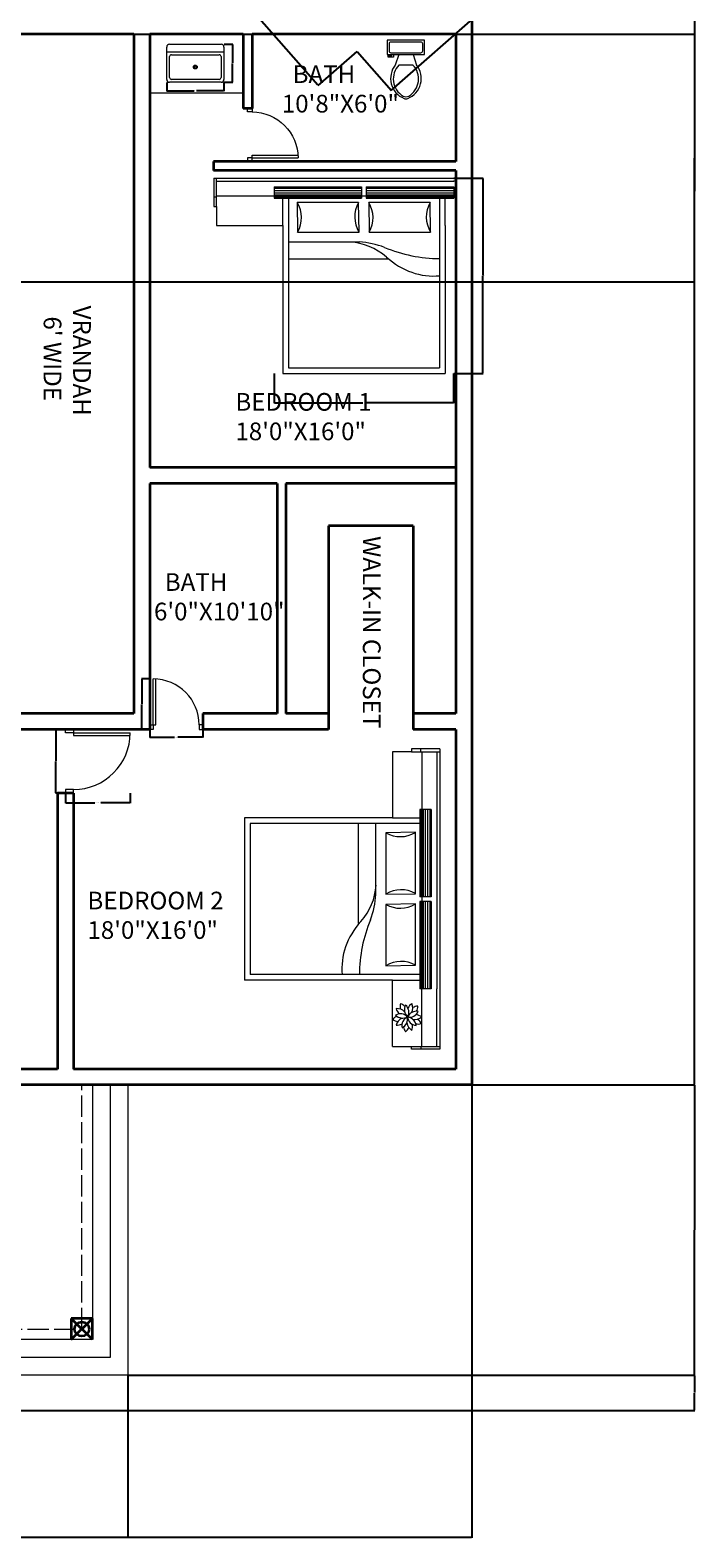
# Model space of a CAD drawing. Units: inches. Extents: x 4602 to 5612, y 5125 to 6591.
# Tile 3 of 6: x 5237 to 5612, y 5125 to 5977. Entities that reach past the tile are written whole.
import ezdxf

# ---------------------------------------------------------------- set-up
doc = ezdxf.new("R2010")
doc.units = ezdxf.units.IN
doc.linetypes.add('ACAD_ISO02W100', pattern=[15, 12, -3])
for name, color, linetype, lineweight in [('A-ANNO-DIMS', 2, 'Continuous', 18), ('A-AREA-IDEN', 7, 'Continuous', 18), ('A-COLS', 7, 'Continuous', 35), ('A-DOOR', 4, 'Continuous', 18), ('A-FLOR-CASE', 9, 'Continuous', 18), ('A-FLOR-EDGE', 7, 'Continuous', 18), ('A-FLOR-FIXT', 8, 'Continuous', 18), ('A-FLOR-OVHD', 8, 'ACAD_ISO02W100', 13), ('A-FLOR-STRS', 7, 'Continuous', 18), ('A-FURN', 8, 'Continuous', 13), ('A-WALL', 7, 'Continuous', 35)]:
    doc.layers.add(name, color=color, linetype=linetype, lineweight=lineweight)
doc.styles.add('ATTR', font='romans.shx', dxfattribs={"width": 0.8, "height": 1.075})
doc.styles.get("Standard").update_dxf_attribs({"font": 'arial.ttf'})
doc.dimstyles.get("Standard").update_dxf_attribs({"dimtxt": 0.18, "dimasz": 0.18, "dimexe": 0.18, "dimexo": 0.0625, "dimgap": 0.09, "dimtad": 0, "dimtih": 1, "dimtoh": 1, "dimdec": 4, "dimzin": 0, "dimdsep": 46, "dimtxsty": 'Standard', "dimcen": 0.09, "dimadec": 0, "dimazin": 0, "dimtfac": 1, "dimtdec": 4, "dimtofl": 0, "dimtmove": 0, "dimatfit": 3, "dimfxl": 1, "dimtolj": 1, "dimtzin": 0, "dimarcsym": 0})

# ---------------------------------------------------------------- blocks, each defined once
blk = doc.blocks.new('A$C25213C04')
for p, q in [((961, 2561), (805, 2831)), ((2063, 2927, 1584), (1415, 2360, 1584)), ((2063, 2927, 1584), (3697, 1495, 1584)), ((961, 2590), (805, 2320)), ((936, 2575), (1248, 2575)), ((2506, 2330, 1584), (2338, 2162, 1584)), ((2306, 2131, 1584), (2256, 2081, 1584)), ((3178, 1881), (3005, 2048)), ((2140, 1966, 1584), (2022, 1849, 1584)), ((1493, 1691), (720, 773)), ((2411, 918), (1493, 1691)), ((3026, 1811, 1584), (2854, 1589, 1584)), ((2839, 1570, 1584), (2748, 1452, 1584)), ((3697, 1495, 1584), (3220, 778, 1584)), ((2708, 1401, 1584), (2653, 1329, 1584)), ((3783, 1288), (3260, 764)), ((3783, 1245), (3302, 764)), ((4207, 863), (3783, 1288)), ((4165, 863), (3783, 1245)), ((720, 773), (1638, 0)), ((1638, 0), (2411, 918)), ((3260, 764), (3684, 340)), ((3302, 764), (3684, 382)), ((3684, 340), (4207, 863)), ((3684, 382), (4165, 863))]:
    blk.add_line(p, q)
at = {"linetype": 'ByBlock'}
for p, q in [((133, 1730), (136, 1691)), ((896, 1561), (877, 1527))]:
    blk.add_line(p, q, dxfattribs=at)
blk.add_lwpolyline([(725, 2173, -0.232884), (950, 2110, -0.135002), (887, 1960, -0.190823), (579, 2053, -0.215879), (600, 2250, -0.243587), (764, 2155, 4.263709)], format="xyb")
blk.add_lwpolyline([(472, 697, 0.343499), (533, 723, 0.070096), (548, 767, -0.063818), (573, 843, 0.079553), (601, 928, -0.057815), (620, 1007, 0.080725), (637, 1068, 0.324043), (600, 1120, -0.019241), (459, 1179, 0.08432), (309, 1223, -0.023422), (183, 1248, 0.070372), (146, 1253, 0.295986), (100, 1217, 0.032258), (86, 1168, -0.067929), (60, 1097, 0.081366), (35, 1016, -0.070774), (15, 936, 0.059814), (0, 885, 0.300433), (27, 833, 0.039992), (72, 815, -0.020153), (147, 783, 0.038402), (259, 739, 0.019707), (344, 722, -0.015856), (435, 705, 0.018827), (472, 697, 1.060826)], format="xyb", dxfattribs=at)
at = {"linetype": 'ByBlock', "flags": 128}
blk.add_lwpolyline([(324, 993, -1), (314, 960, -1)], format="xyb", close=True, dxfattribs=at)
blk.add_circle((953, 2575), 250)
for centre, radius, start, end in [((6904, 6804, 1584), 6250, 218.7122, 226.8714), ((6904, 6804, 1584), 6246, 218.7173, 226.8972), ((2075, 2768, 1584), 34.6, 301.5027, 35.2471), ((3283, 3449, 1584), 1352, 209.2555, 217.5058), ((2031, 2594, 1584), 222, 173.7702, 227.3147), ((1881, 2465, 1584), 169, 60.105, 114.9918), ((2065, 2440, 1584), 217, 75.8217, 128.2602), ((435, 4670, 1584), 2546, 306.4044, 310.6458), ((2178, 2539, 1584), 222, 167.7702, 221.3147), ((2015, 2427, 1584), 169, 54.105, 108.9918), ((2196, 2383, 1584), 217, 69.8217, 122.2602), ((1856, 2548, 1584), 282, 8.7006, 21.3114), ((1999, 2512, 1584), 282, 333.4414, 15.3114), ((742, 2652), 470, 213.6928, 250.0667), ((-111, -1286), 3707, 72.7192, 82.835), ((435, 4670, 1584), 2546, 293.2711, 302.9022), ((908, 3983, 1584), 1733, 288.4557, 300.3041), ((1986, 2631, 1584), 226, 242.3583, 273.8129), ((1838, 2738, 1584), 282, 280.859, 296.2171), ((2136, 2581, 1584), 226, 236.3583, 300.7775), ((1993, 2688, 1584), 282, 280.859, 322.7291), ((2044, 2704, 1584), 282, 271.8903, 313.7604), ((7978, 8701, 1584), 8396, 227.9717, 230.3292), ((-1544, 2942), 2094, 323.3441, 341.8043), ((590, 2045), 206, 32.2825, 87.042), ((742, 2652), 470, 270.1213, 301.8614), ((12303, 12967, 1584), 15201, 224.2521, 233.3075), ((3562, 3960, 1584), 2657, 217.5941, 222.0435), ((2720, 1975, 1584), 282, 105.7877, 147.6577), ((2508, 2077, 1584), 217, 358.839, 51.2774), ((591, 1710), 371, 44.935, 87.2084), ((487, 1559), 554, 48.4222, 73.8484), ((773, 1914), 264, 47.9991, 100.4376), ((2708, 2129, 1584), 226, 180.3216, 244.7408), ((2862, 2114, 1584), 282, 167.3388, 209.2088), ((2874, 2061, 1584), 282, 158.3701, 200.2401), ((6904, 6804, 1584), 6246, 227.5711, 228.2803), ((6904, 6804, 1584), 6250, 227.7194, 228.2519), ((2639, 1946, 1584), 169, 12.1073, 66.9941), ((7978, 8701, 1584), 8396, 231.1014, 231.3893), ((2825, 1872, 1584), 282, 99.7877, 112.3986), ((2625, 1995, 1584), 217, 352.839, 45.2774), ((2930, 1759, 1584), 282, 99.7877, 112.3986), ((6904, 6804, 1584), 6246, 229.2463, 229.7871), ((6904, 6804, 1584), 6250, 229.3273, 229.7524), ((8643, 8118, 1584), 8396, 226.2108, 226.4615), ((2730, 1883, 1584), 217, 352.839, 45.2774), ((10966, 12498, 1584), 13958, 229.1973, 231.6399), ((2651, 2143, 1584), 222, 259.7845, 313.329), ((2829, 2026, 1584), 226, 207.2862, 238.7408), ((2774, 2046, 1584), 222, 253.7845, 307.329), ((2997, 1955, 1584), 282, 184.882, 200.2401), ((2741, 1851, 1584), 169, 6.1073, 60.9941), ((6904, 6804, 1584), 6246, 230.2513, 238.8423), ((6904, 6804, 1584), 6250, 230.3855, 238.8474), ((2846, 1738, 1584), 169, 6.1073, 60.9941), ((8643, 8118, 1584), 8396, 227.1305, 229.5879), ((2934, 1914, 1584), 226, 201.8609, 238.7408), ((2879, 1934, 1584), 222, 253.7845, 307.329), ((3102, 1842, 1584), 282, 184.882, 200.2401), ((3294, 1377, 1584), 282, 82.2482, 124.1182), ((3140, 1555, 1584), 217, 335.2995, 27.7379), ((12014, 11580, 1584), 13958, 225.9197, 228.3623), ((3345, 1523, 1584), 226, 156.7821, 221.2013), ((3469, 1394, 1584), 282, 134.8306, 176.7006), ((3479, 1447, 1584), 282, 143.7993, 185.6693), ((3207, 1382, 1584), 169, 348.5678, 43.4546), ((3349, 1240, 1584), 282, 76.2482, 88.8591), ((4054, 2773, 1584), 1352, 240.0538, 248.3041), ((3214, 1433, 1584), 217, 329.2995, 21.7379), ((5640, 111, 1584), 2546, 146.9138, 151.1553), ((3538, 1486, 1584), 34.6, 62.3126, 156.0569), ((3298, 1558, 1584), 222, 236.2449, 289.7895), ((3414, 1380, 1584), 226, 183.7467, 215.2013), ((3539, 1247, 1584), 282, 161.3425, 176.7006), ((3263, 1255, 1584), 169, 342.5678, 37.4546), ((5640, 111, 1584), 2546, 154.6574, 164.2885), ((4896, 489, 1584), 1733, 157.2556, 169.1039), ((3372, 1420, 1584), 222, 230.2449, 283.7895), ((4524, 3117, 1584), 2657, 235.5161, 239.9655)]:
    blk.add_arc(centre, radius, start, end)
at = {"linetype": 'ByBlock'}
for centre, radius, start, end in [((3117, 1104), 3051, 155.0292, 167.8975), ((-2061, 2301), 3051, 346.2024, 359.1081), ((4037, 1940), 3187, 175.3548, 175.9684), ((4037, 1940), 3187, 179.6641, 187.4345), ((168, 1736), 35.5, 167.4303, 189.0652), ((187, 1686), 51, 173.5933, 247.766), ((1112, 4418), 2936, 251.2253, 257.771), ((1098, 4417), 2932, 258.0523, 264.7029), ((826, 1556), 57.8, 270.4071, 330.8661), ((867, 1581), 35.5, 325.0347, 346.6697), ((280, 872), 108, 80.0068, 116.3761), ((349, 1084), 108, 207.805, 244.1743), ((212, 1006), 108, 297.805, 334.1743), ((215, 1016), 108, 350.0068, 26.3761), ((424, 937), 108, 170.0068, 206.3761), ((427, 947), 108, 117.805, 154.1743), ((290, 869), 108, 27.805, 64.1743), ((358, 1081), 108, 260.0068, 296.3761)]:
    blk.add_arc(centre, radius, start, end, dxfattribs=at)
for major_axis, start_param, end_param in [((-153, 153), 3.927057, 7.06865), ((-64.8, 64.8), 3.927057, 7.06865), ((-153, 153), 0.785465, 3.927057), ((-64.8, 64.8), 0.785465, 3.927057)]:
    blk.add_ellipse((953, 2575), major_axis=major_axis, ratio=1, start_param=start_param, end_param=end_param)
blk = doc.blocks.new("30'' Sink Single PV")
blk.add_line((-15, -3.999996), (15, -3.999996))
for points in [[(-13.5, 0), (13.5, 0)], [(-15, -18.499996), (-15, -1.5)], [(-13.5, -17.499996), (-13.5, -6.499996)], [(-12.5, -5.499996), (12.5, -5.499996)], [(13.5, -6.499996), (13.5, -17.499996)], [(15, -1.5), (15, -18.499996)], [(13.5, -19.999996), (-13.5, -19.999996)], [(12.5, -18.499996), (-12.5, -18.499996)]]:
    blk.add_lwpolyline(points)
for radius in [1, 0.5]:
    blk.add_circle((0, -11.999996), radius)
for centre, radius, start, end in [((-13.5, -1.5), 1.5, 90, 180), ((-12.5, -6.499996), 1, 90, 180), ((12.5, -6.499996), 1, 0, 90), ((13.5, -1.5), 1.5, 0, 90), ((-13.5, -18.499996), 1.5, 180, 270), ((-12.5, -17.499996), 1, 180, 270), ((12.5, -17.499996), 1, 270, 0), ((13.5, -18.499996), 1.5, 270, 0)]:
    blk.add_arc(centre, radius, start, end)
at = {"style": 'ATTR', "width": 0.8, "flags": 9}
blk.add_attdef('ESTCODE', (0, 0), '', height=0.006, dxfattribs=at)
blk = doc.blocks.new('*U9')
for p, q in [((-254, -216), (-203, -216)), ((-254, -241), (-254, -216)), ((-203, -216), (-203, -203)), ((-178, -203), (-178, -241)), ((-102, -203), (-152, -356)), ((102, -203), (152, -356)), ((241, -152), (241, -51)), ((-178, -241), (-254, -241)), ((102, -356), (-102, -356))]:
    blk.add_line(p, q)
blk.add_lwpolyline([(267, -203), (267, 0), (-267, 0), (-267, -203)], close=True)
for points in [[(-241, -51), (-241, -152)], [(216, -25), (-216, -25)], [(-216, -178), (216, -178)]]:
    blk.add_lwpolyline(points)
for centre, radius, start, end in [((-219, -48), 22.5, 81.8699, 188.1301), ((-219, -156), 22.5, 171.8699, 278.1301), ((219, -48), 22.5, 351.8699, 98.1301), ((219, -156), 22.5, 261.8699, 8.1301), ((89, -548), 309, 141.4691, 247.9714), ((107, -554), 288, 136.3677, 238.9468), ((-89, -548), 309, 292.0284, 38.5307), ((-107, -554), 288, 301.053, 43.6321), ((0, -708), 102, 245.7318, 294.2682), ((0, -737), 102, 254.8605, 285.1395)]:
    blk.add_arc(centre, radius, start, end)
blk = doc.blocks.new('A$C7BDD1693')
for p, q in [((0, 2.068), (0, 1.768)), ((0, 2.068), (1.615, 2.068)), ((0.03, 1.768), (0.03, 2.068)), ((0.03, 2.038), (0.64, 2.038)), ((0.64, 2.038), (1.565, 2.038)), ((0.64, 1.978), (1.565, 1.978)), ((0.64, 1.978), (0.64, 1.858)), ((0.64, 1.963), (1.565, 1.963)), ((0.64, 1.937), (1.565, 1.937)), ((1.565, 2.038), (1.615, 2.038)), ((1.565, 1.978), (1.565, 1.858)), ((1.615, 2.068), (2.54, 2.068)), ((1.615, 2.038), (2.54, 2.038)), ((1.615, 1.978), (1.615, 1.858)), ((1.615, 1.978), (2.54, 1.978)), ((1.615, 1.963), (2.54, 1.963)), ((1.615, 1.937), (2.54, 1.937)), ((2.54, 2.068), (3.18, 2.068)), ((3.15, 2.038), (2.54, 2.038)), ((2.54, 1.978), (2.54, 1.858)), ((3.15, 1.768), (3.15, 2.068)), ((3.18, 2.068), (3.18, 1.768)), ((0.03, 1.868), (0, 1.868)), ((0, 1.768), (0.03, 1.768)), ((0.03, 1.88), (0.64, 1.88)), ((0.03, 1.768), (0.03, 1.568)), ((0.03, 1.768), (0.03, 1.568)), ((0.64, 1.912), (1.565, 1.912)), ((0.64, 1.893), (1.565, 1.893)), ((0.64, 1.877), (1.565, 1.877)), ((0.64, 1.866), (1.565, 1.866)), ((0.64, 1.858), (1.565, 1.858)), ((0.73, 1.568), (0.73, 1.858)), ((0.79, 1.858), (0.79, 0.06)), ((1.533, 1.81), (0.883, 1.81)), ((0.883, 1.81), (0.887, 1.498)), ((1.537, 1.498), (1.533, 1.81)), ((1.565, 1.88), (1.615, 1.88)), ((1.615, 1.912), (2.54, 1.912)), ((1.615, 1.893), (2.54, 1.893)), ((1.615, 1.877), (2.54, 1.877)), ((1.615, 1.866), (2.54, 1.866)), ((1.615, 1.858), (2.54, 1.858)), ((2.291, 1.81), (1.641, 1.81)), ((1.641, 1.81), (1.646, 1.498)), ((2.296, 1.498), (2.291, 1.81)), ((2.39, 1.858), (2.39, 0.06)), ((2.45, 1.568), (2.45, 1.858)), ((3.15, 1.88), (2.54, 1.88)), ((3.15, 1.868), (3.18, 1.868)), ((3.15, 1.568), (3.15, 1.768)), ((3.18, 1.768), (3.15, 1.768)), ((0.03, 1.568), (0.73, 1.568)), ((0.73, 1.568), (0.73, 0)), ((0.887, 1.498), (1.537, 1.498)), ((1.646, 1.498), (2.296, 1.498)), ((3.15, 1.568), (2.45, 1.568)), ((2.45, 1.568), (2.45, 0)), ((1.54, 1.392), (0.79, 1.392)), ((1.848, 1.209), (0.79, 1.209)), ((0.73, 0), (2.45, 0)), ((0.79, 0.06), (2.39, 0.06))]:
    blk.add_line(p, q)
for centre, radius, start, end in [((0.626, 1.65), 0.303, 329.8722, 31.8713), ((1.794, 1.658), 0.303, 149.8722, 211.8713), ((1.384, 1.65), 0.303, 329.8722, 31.8713), ((2.553, 1.658), 0.303, 149.8722, 211.8713), ((2.74, 1.667), 0.115, 63.1324, 112.6013), ((2.798, 1.845), 0.125, 215.1301, 245.4931), ((2.879, 1.849), 0.155, 184.2105, 205.3514), ((2.726, 1.74), 0.0968, 57.5086, 91.2476), ((2.884, 1.823), 0.106, 170.7761, 244.5159), ((2.743, 1.749), 0.098, 347.0447, 68.2473), ((2.938, 1.802), 0.125, 143.1301, 173.4932), ((2.751, 1.802), 0.115, 351.1324, 40.6013), ((2.944, 1.713), 0.106, 98.7761, 172.5159), ((2.83, 1.825), 0.098, 275.0447, 356.2473), ((2.967, 1.726), 0.155, 112.2105, 133.3514), ((2.883, 1.833), 0.115, 279.1324, 328.6013), ((2.817, 1.838), 0.0968, 345.5086, 19.2476), ((2.941, 1.655), 0.125, 71.1301, 101.4931), ((2.791, 1.624), 0.0968, 129.5086, 163.2476), ((2.735, 1.803), 0.155, 256.2105, 277.3514), ((2.788, 1.643), 0.098, 59.0447, 140.2473), ((2.761, 1.8), 0.106, 242.7761, 316.5159), ((2.865, 1.615), 0.115, 135.1324, 184.6013), ((2.713, 1.725), 0.125, 287.1301, 317.4932), ((2.903, 1.653), 0.098, 131.0447, 212.2473), ((2.745, 1.676), 0.106, 314.7761, 28.5159), ((2.921, 1.65), 0.0968, 201.5086, 235.2476), ((2.858, 1.622), 0.106, 26.7761, 100.5159), ((2.929, 1.765), 0.098, 203.0447, 284.2473), ((2.953, 1.718), 0.115, 207.1324, 256.6013), ((2.734, 1.652), 0.155, 328.2105, 349.3514), ((2.802, 1.607), 0.125, 359.1301, 29.4932), ((2.937, 1.782), 0.0968, 273.5086, 307.2476), ((2.877, 1.605), 0.155, 40.2105, 61.3514)]:
    blk.add_arc(centre, radius, start, end)
for centre, major_axis, ratio, start_param, end_param in [((1.413, 0.552), (0, -0.842), 0.84, 2.512571, 3.097265), ((1.474, 0.023), (0, -1.371), 0.84, 2.845884, 3.083884), ((2.394, 3.329), (0, -2.112), 0.84, -0.336035, -0.002349), ((2.261, 1.856), (0.259, -0.793), 0.868451, -0.988378, -0.183496)]:
    blk.add_ellipse(centre, major_axis=major_axis, ratio=ratio, start_param=start_param, end_param=end_param)
blk = doc.blocks.new('DOOR-36IN-DEEP-JAMB')
for p, q in [((2, 4.5), (2, 36.5)), ((3.5, 4.5), (3.5, 36.46)), ((0, 4.5), (2, 4.5)), ((2, 4.5), (2, 0)), ((2, 4.5), (3.5, 4.5)), ((36, 4.5), (34, 4.5)), ((34, 4.5), (34, 0)), ((2, 0), (0, 0)), ((34, 0), (36, 0))]:
    blk.add_line(p, q)
blk.add_arc((2, 4.5), 32, 0, 90)
blk = doc.blocks.new('DOOR-30IN')
for p, q in [((26, 30), (26, 28)), ((26, 28), (28.5, 28)), ((28.5, 28), (28.5, 30)), ((26, 2), (0, 2)), ((26, 3.5), (0.04, 3.5)), ((26, 2), (26, 3.5)), ((26, 0), (26, 2)), ((26, 2), (28.5, 2)), ((28.5, 2), (28.5, 0))]:
    blk.add_line(p, q)
blk.add_arc((26, 2), 26, 90, 180)
blk = doc.blocks.new('POST-POOMUKHAM')
for p, q in [((12, 12), (0, 12)), ((0, 12), (0, 0)), ((12, 0), (0, 12)), ((0, 0), (12, 12)), ((12, 0), (12, 12))]:
    blk.add_line(p, q)
blk.add_circle((6, 6), 4.06)
blk = doc.blocks.new('BED-DOUBLE')
for p, q in [((0, 108.76), (49.36, 108.76)), ((0, 105.55), (49.36, 105.55)), ((0, 105.55), (0, 99.15)), ((0, 104.75), (49.36, 104.75)), ((0, 103.35), (49.36, 103.35)), ((49.36, 108.76), (52.03, 108.76)), ((49.36, 105.55), (49.36, 99.15)), ((52.03, 110.36), (101.4, 110.36)), ((52.03, 108.76), (101.4, 108.76)), ((52.03, 105.55), (52.03, 99.15)), ((52.03, 105.55), (101.4, 105.55)), ((52.03, 104.75), (101.4, 104.75)), ((52.03, 103.35), (101.4, 103.35)), ((101.4, 105.55), (101.4, 99.15)), ((0, 102.06), (49.36, 102.06)), ((0, 101), (49.36, 101)), ((0, 100.18), (49.36, 100.18)), ((0, 99.59), (49.36, 99.59)), ((0, 99.15), (49.36, 99.15)), ((4.8, 83.67), (4.8, 99.15)), ((8.01, 99.15), (8.01, 3.2)), ((47.64, 96.58), (12.95, 96.58)), ((12.95, 96.58), (13.21, 79.95)), ((47.9, 79.95), (47.64, 96.58)), ((49.36, 100.32), (52.03, 100.32)), ((52.03, 102.06), (101.4, 102.06)), ((52.03, 101), (101.4, 101)), ((52.03, 100.18), (101.4, 100.18)), ((52.03, 99.59), (101.4, 99.59)), ((52.03, 99.15), (101.4, 99.15)), ((88.11, 96.58), (53.42, 96.58)), ((53.42, 96.58), (53.67, 79.95)), ((88.36, 79.95), (88.11, 96.58)), ((93.39, 99.15), (93.39, 3.2)), ((96.59, 83.67), (96.59, 99.15)), ((4.8, 83.67), (4.8, 0)), ((13.21, 79.95), (47.9, 79.95)), ((53.67, 79.95), (88.36, 79.95)), ((96.59, 83.67), (96.59, 0)), ((48.03, 74.3), (8.01, 74.3)), ((64.45, 64.53), (8.01, 64.53)), ((4.8, 0), (96.59, 0)), ((8.01, 3.2), (93.39, 3.2))]:
    blk.add_line(p, q)
for centre, start, end in [((-0.76, 88.06), 329.87223, 31.87128), ((61.61, 88.48), 149.87223, 211.87128), ((39.71, 88.06), 329.87223, 31.87128), ((102.07, 88.48), 149.87223, 211.87128)]:
    blk.add_arc(centre, 16.15, start, end)
for centre, major_axis, ratio, start_param, end_param in [((41.23, 29.43), (0, -44.91), 0.84, 2.512571, 3.097265), ((44.48, 1.25), (0, -73.18), 0.84, 2.845884, 3.083884), ((93.61, 177.65), (0, -112.7), 0.84, -0.336035, -0.002349), ((86.52, 99.05), (13.81, -42.31), 0.868451, -0.988378, -0.183496)]:
    blk.add_ellipse(centre, major_axis=major_axis, ratio=ratio, start_param=start_param, end_param=end_param)
blk = doc.blocks.new('*D23')
at = {"layer": 'A-ANNO-DIMS', "color": 0, "lineweight": -2, "transparency": 16777216}
for p, q in [((5256.74, 5545.49), (5256.74, 5539.9)), ((5256.92, 5540.08), (5273.3, 5540.08)), ((5293.06, 5540.08), (5276.68, 5540.08)), ((5293.24, 5545.49), (5293.24, 5539.9))]:
    blk.add_line(p, q, dxfattribs=at)
at = {"layer": 'A-ANNO-DIMS', "color": 0, "transparency": 16777216}
for points in [[(5256.92, 5540.11), (5256.92, 5540.05), (5256.74, 5540.08)], [(5293.06, 5540.11), (5293.06, 5540.05), (5293.24, 5540.08)]]:
    blk.add_solid(points, dxfattribs=at)
at = {"layer": 'Defpoints', "color": 0, "transparency": 16777216}
for p in [(5256.74, 5545.55), (5293.24, 5545.55), (5293.24, 5540.08)]:
    blk.add_point(p, dxfattribs=at)
at = {"layer": 'A-ANNO-DIMS', "color": 0, "transparency": 16777216, "insert": (5274.99, 5540.08), "char_height": 0.18, "attachment_point": 5}
blk.add_mtext('\\A1;DEEP-JAMB DOOR 37 TYP.', dxfattribs=at)
blk = doc.blocks.new('*D24')
at = {"layer": 'A-ANNO-DIMS', "color": 0, "lineweight": -2, "transparency": 16777216}
for p, q in [((5256.68, 5581.55), (5251.08, 5581.55)), ((5251.26, 5581.37), (5251.26, 5563.73)), ((5251.26, 5545.73), (5251.26, 5563.37)), ((5256.68, 5545.55), (5251.08, 5545.55))]:
    blk.add_line(p, q, dxfattribs=at)
at = {"layer": 'A-ANNO-DIMS', "color": 0, "transparency": 16777216}
for points in [[(5251.23, 5581.37), (5251.29, 5581.37), (5251.26, 5581.55)], [(5251.23, 5545.73), (5251.29, 5545.73), (5251.26, 5545.55)]]:
    blk.add_solid(points, dxfattribs=at)
at = {"layer": 'Defpoints', "color": 0, "transparency": 16777216}
for p in [(5256.74, 5581.55), (5251.26, 5545.55), (5256.74, 5545.55)]:
    blk.add_point(p, dxfattribs=at)
at = {"layer": 'A-ANNO-DIMS', "color": 0, "transparency": 16777216, "insert": (5251.26, 5563.55), "char_height": 0.18, "attachment_point": 5}
blk.add_mtext('\\A1;36 TYP.', dxfattribs=at)
blk = doc.blocks.new('*D27')
at = {"layer": 'A-ANNO-DIMS', "color": 0, "lineweight": -2, "transparency": 16777216}
for p, q in [((5304.24, 5581.49), (5304.24, 5576.87)), ((5304.42, 5577.05), (5318.3, 5577.05)), ((5334.06, 5577.05), (5320.17, 5577.05)), ((5334.24, 5581.49), (5334.24, 5576.87))]:
    blk.add_line(p, q, dxfattribs=at)
at = {"layer": 'A-ANNO-DIMS', "color": 0, "transparency": 16777216}
for points in [[(5304.42, 5577.08), (5304.42, 5577.02), (5304.24, 5577.05)], [(5334.06, 5577.08), (5334.06, 5577.02), (5334.24, 5577.05)]]:
    blk.add_solid(points, dxfattribs=at)
at = {"layer": 'Defpoints', "color": 0, "transparency": 16777216}
for p in [(5304.24, 5581.55), (5334.24, 5581.55), (5334.24, 5577.05)]:
    blk.add_point(p, dxfattribs=at)
at = {"layer": 'A-ANNO-DIMS', "color": 0, "transparency": 16777216, "insert": (5319.24, 5577.05), "char_height": 0.18, "attachment_point": 5}
blk.add_mtext('\\A1;DOOR 30 TYP.', dxfattribs=at)
blk = doc.blocks.new('*D28')
at = {"layer": 'A-ANNO-DIMS', "color": 0, "lineweight": -2, "transparency": 16777216}
for p, q in [((5304.18, 5610.05), (5299.56, 5610.05)), ((5299.74, 5609.87), (5299.74, 5595.98)), ((5299.74, 5581.73), (5299.74, 5595.62)), ((5304.18, 5581.55), (5299.56, 5581.55))]:
    blk.add_line(p, q, dxfattribs=at)
at = {"layer": 'A-ANNO-DIMS', "color": 0, "transparency": 16777216}
for points in [[(5299.71, 5609.87), (5299.77, 5609.87), (5299.74, 5610.05)], [(5299.71, 5581.73), (5299.77, 5581.73), (5299.74, 5581.55)]]:
    blk.add_solid(points, dxfattribs=at)
at = {"layer": 'Defpoints', "color": 0, "transparency": 16777216}
for p in [(5304.24, 5610.05), (5299.74, 5581.55), (5304.24, 5581.55)]:
    blk.add_point(p, dxfattribs=at)
at = {"layer": 'A-ANNO-DIMS', "color": 0, "transparency": 16777216, "insert": (5299.74, 5595.8), "char_height": 0.18, "attachment_point": 5}
blk.add_mtext('\\A1;29 TYP.', dxfattribs=at)
blk = doc.blocks.new('*D37')
at = {"layer": 'A-ANNO-DIMS', "color": 0, "lineweight": -2, "transparency": 16777216}
for p, q in [((5476.11, 5893.1), (5492.78, 5893.1)), ((5492.6, 5892.92), (5492.6, 5838.11)), ((5492.6, 5782.93), (5492.6, 5837.74)), ((5476.11, 5782.75), (5492.78, 5782.75))]:
    blk.add_line(p, q, dxfattribs=at)
at = {"layer": 'A-ANNO-DIMS', "color": 0, "transparency": 16777216}
for points in [[(5492.57, 5892.92), (5492.63, 5892.92), (5492.6, 5893.1)], [(5492.57, 5782.93), (5492.63, 5782.93), (5492.6, 5782.75)]]:
    blk.add_solid(points, dxfattribs=at)
at = {"layer": 'Defpoints', "color": 0, "transparency": 16777216}
for p in [(5476.05, 5893.1), (5492.6, 5893.1), (5476.05, 5782.75)]:
    blk.add_point(p, dxfattribs=at)
at = {"layer": 'A-ANNO-DIMS', "color": 0, "transparency": 16777216, "insert": (5492.6, 5837.92), "char_height": 0.18, "attachment_point": 5}
blk.add_mtext('\\A1;DOUBLE BED 110 TYP.', dxfattribs=at)
blk = doc.blocks.new('*D38')
at = {"layer": 'A-ANNO-DIMS', "color": 0, "lineweight": -2, "transparency": 16777216}
for p, q in [((5374.65, 5782.68), (5374.65, 5766.01)), ((5476.05, 5782.68), (5476.05, 5766.01)), ((5374.83, 5766.19), (5424.76, 5766.19)), ((5475.87, 5766.19), (5425.94, 5766.19))]:
    blk.add_line(p, q, dxfattribs=at)
at = {"layer": 'A-ANNO-DIMS', "color": 0, "transparency": 16777216}
for points in [[(5374.83, 5766.22), (5374.83, 5766.16), (5374.65, 5766.19)], [(5475.87, 5766.22), (5475.87, 5766.16), (5476.05, 5766.19)]]:
    blk.add_solid(points, dxfattribs=at)
at = {"layer": 'Defpoints', "color": 0, "transparency": 16777216}
for p in [(5374.65, 5782.75), (5476.05, 5782.75), (5476.05, 5766.19)]:
    blk.add_point(p, dxfattribs=at)
at = {"layer": 'A-ANNO-DIMS', "color": 0, "transparency": 16777216, "insert": (5425.35, 5766.19), "char_height": 0.18, "attachment_point": 5}
blk.add_mtext('\\A1;101 TYP.', dxfattribs=at)
blk = doc.blocks.new('*D43')
at = {"layer": 'A-ANNO-DIMS', "color": 0, "lineweight": -2, "transparency": 16777216}
for p, q in [((5313.85, 5947.25), (5313.85, 5942.28)), ((5314.03, 5942.46), (5329.4, 5942.46)), ((5346.01, 5942.46), (5330.65, 5942.46)), ((5346.19, 5947.25), (5346.19, 5942.28))]:
    blk.add_line(p, q, dxfattribs=at)
at = {"layer": 'A-ANNO-DIMS', "color": 0, "transparency": 16777216}
for points in [[(5314.03, 5942.49), (5314.03, 5942.43), (5313.85, 5942.46)], [(5346.01, 5942.49), (5346.01, 5942.43), (5346.19, 5942.46)]]:
    blk.add_solid(points, dxfattribs=at)
at = {"layer": 'Defpoints', "color": 0, "transparency": 16777216}
for p in [(5313.85, 5947.31), (5346.19, 5947.31), (5346.19, 5942.46)]:
    blk.add_point(p, dxfattribs=at)
at = {"layer": 'A-ANNO-DIMS', "color": 0, "transparency": 16777216, "insert": (5330.02, 5942.46), "char_height": 0.18, "attachment_point": 5}
blk.add_mtext('\\A1;BASIN 32', dxfattribs=at)
blk = doc.blocks.new('*D44')
at = {"layer": 'A-ANNO-DIMS', "color": 0, "lineweight": -2, "transparency": 16777216}
for p, q in [((5346.25, 5968.87), (5351.22, 5968.87)), ((5351.04, 5968.69), (5351.04, 5958.27)), ((5351.04, 5947.49), (5351.04, 5957.91)), ((5346.25, 5947.31), (5351.22, 5947.31))]:
    blk.add_line(p, q, dxfattribs=at)
at = {"layer": 'A-ANNO-DIMS', "color": 0, "transparency": 16777216}
for points in [[(5351.01, 5968.69), (5351.07, 5968.69), (5351.04, 5968.87)], [(5351.01, 5947.49), (5351.07, 5947.49), (5351.04, 5947.31)]]:
    blk.add_solid(points, dxfattribs=at)
at = {"layer": 'Defpoints', "color": 0, "transparency": 16777216}
for p in [(5346.19, 5968.87), (5351.04, 5968.87), (5346.19, 5947.31)]:
    blk.add_point(p, dxfattribs=at)
at = {"layer": 'A-ANNO-DIMS', "color": 0, "transparency": 16777216, "insert": (5351.04, 5958.09), "char_height": 0.18, "attachment_point": 5}
blk.add_mtext('\\A1;22', dxfattribs=at)
blk = doc.blocks.new('*D49')
at = {"layer": 'A-ANNO-DIMS', "color": 0, "lineweight": -2, "transparency": 16777216}
for p, q in [((5293.01, 6111.54), (5270.91, 6092.21)), ((5271.16, 6092.19), (5335.08, 6019.13)), ((5399.32, 5945.7), (5335.4, 6018.76)), ((5421.4, 5964.78), (5399.3, 5945.45))]:
    blk.add_line(p, q, dxfattribs=at)
at = {"layer": 'A-ANNO-DIMS', "color": 0, "transparency": 16777216}
for points in [[(5271.18, 6092.21), (5271.14, 6092.17), (5271.04, 6092.33)], [(5399.34, 5945.72), (5399.29, 5945.68), (5399.43, 5945.57)]]:
    blk.add_solid(points, dxfattribs=at)
at = {"layer": 'Defpoints', "color": 0, "transparency": 16777216}
for p in [(5293.05, 6111.58), (5421.45, 5964.83), (5399.43, 5945.57)]:
    blk.add_point(p, dxfattribs=at)
at = {"layer": 'A-ANNO-DIMS', "color": 0, "transparency": 16777216, "insert": (5335.24, 6018.95), "char_height": 0.18, "attachment_point": 5}
blk.add_mtext('\\A1;FAMILY SEATING 195', dxfattribs=at)
blk = doc.blocks.new('*D50')
at = {"layer": 'A-ANNO-DIMS', "color": 0, "lineweight": -2, "transparency": 16777216}
for p, q in [((5523.54, 6054.06), (5542.88, 6031.96)), ((5542.62, 6031.97), (5491.94, 5987.63)), ((5440.84, 5942.93), (5491.53, 5987.27)), ((5421.49, 5964.78), (5440.83, 5942.68))]:
    blk.add_line(p, q, dxfattribs=at)
at = {"layer": 'A-ANNO-DIMS', "color": 0, "transparency": 16777216}
for points in [[(5542.6, 6032), (5542.64, 6031.95), (5542.76, 6032.09)], [(5440.82, 5942.95), (5440.86, 5942.91), (5440.71, 5942.81)]]:
    blk.add_solid(points, dxfattribs=at)
at = {"layer": 'Defpoints', "color": 0, "transparency": 16777216}
for p in [(5523.5, 6054.11), (5542.76, 6032.09), (5421.45, 5964.83)]:
    blk.add_point(p, dxfattribs=at)
at = {"layer": 'A-ANNO-DIMS', "color": 0, "transparency": 16777216, "insert": (5491.73, 5987.45), "char_height": 0.18, "attachment_point": 5}
blk.add_mtext('\\A1;136', dxfattribs=at)
blk = doc.blocks.new('*D57')
at = {"layer": 'A-ANNO-DIMS', "color": 0, "lineweight": -2, "transparency": 16777216}
for p, q in [((4720.24, 5380.49), (4720.24, 5124.52)), ((5486.24, 5380.49), (5486.24, 5124.52)), ((4720.42, 5124.7), (5102.95, 5124.7)), ((5486.06, 5124.7), (5103.53, 5124.7))]:
    blk.add_line(p, q, dxfattribs=at)
at = {"layer": 'A-ANNO-DIMS', "color": 0, "transparency": 16777216}
for points in [[(4720.42, 5124.73), (4720.42, 5124.67), (4720.24, 5124.7)], [(5486.06, 5124.73), (5486.06, 5124.67), (5486.24, 5124.7)]]:
    blk.add_solid(points, dxfattribs=at)
at = {"layer": 'Defpoints', "color": 0, "transparency": 16777216}
for p in [(4720.24, 5380.55), (5486.24, 5380.55), (5486.24, 5124.7)]:
    blk.add_point(p, dxfattribs=at)
at = {"layer": 'A-ANNO-DIMS', "color": 0, "transparency": 16777216, "insert": (5103.24, 5124.7), "char_height": 0.18, "attachment_point": 5}
blk.add_mtext('\\A1;766', dxfattribs=at)
blk = doc.blocks.new('*D58')
at = {"layer": 'A-ANNO-DIMS', "color": 0, "lineweight": -2, "transparency": 16777216}
for p, q in [((5486.3, 6390.55), (5612.27, 6390.55)), ((5612.09, 6390.37), (5612.09, 5885.73)), ((5612.09, 5380.73), (5612.09, 5885.37)), ((5486.3, 5380.55), (5612.27, 5380.55))]:
    blk.add_line(p, q, dxfattribs=at)
at = {"layer": 'A-ANNO-DIMS', "color": 0, "transparency": 16777216}
for points in [[(5612.06, 6390.37), (5612.12, 6390.37), (5612.09, 6390.55)], [(5612.06, 5380.73), (5612.12, 5380.73), (5612.09, 5380.55)]]:
    blk.add_solid(points, dxfattribs=at)
at = {"layer": 'Defpoints', "color": 0, "transparency": 16777216}
for p in [(5486.24, 6390.55), (5612.09, 6390.55), (5486.24, 5380.55)]:
    blk.add_point(p, dxfattribs=at)
at = {"layer": 'A-ANNO-DIMS', "color": 0, "transparency": 16777216, "insert": (5612.09, 5885.55), "char_height": 0.18, "attachment_point": 5}
blk.add_mtext('\\A1;1010', dxfattribs=at)
blk = doc.blocks.new('*D64')
at = {"layer": 'A-ANNO-DIMS', "color": 0, "lineweight": -2, "transparency": 16777216}
for p, q in [((4860.3, 5974.55), (5612.27, 5974.55)), ((5612.09, 5974.37), (5612.09, 5904.73)), ((5612.09, 5834.73), (5612.09, 5904.37)), ((4860.3, 5834.55), (5612.27, 5834.55))]:
    blk.add_line(p, q, dxfattribs=at)
at = {"layer": 'A-ANNO-DIMS', "color": 0, "transparency": 16777216}
for points in [[(5612.06, 5974.37), (5612.12, 5974.37), (5612.09, 5974.55)], [(5612.06, 5834.73), (5612.12, 5834.73), (5612.09, 5834.55)]]:
    blk.add_solid(points, dxfattribs=at)
at = {"layer": 'Defpoints', "color": 0, "transparency": 16777216}
for p in [(4860.24, 5974.55), (5612.09, 5974.55), (4860.24, 5834.55)]:
    blk.add_point(p, dxfattribs=at)
at = {"layer": 'A-ANNO-DIMS', "color": 0, "transparency": 16777216, "insert": (5612.09, 5904.55), "char_height": 0.18, "attachment_point": 5}
blk.add_mtext('\\A1;140', dxfattribs=at)
blk = doc.blocks.new('*D65')
at = {"layer": 'A-ANNO-DIMS', "color": 0, "lineweight": -2, "transparency": 16777216}
for p, q in [((4914.59, 5216.49), (4914.59, 5124.52)), ((5291.89, 5216.49), (5291.89, 5124.52)), ((4914.77, 5124.7), (5102.85, 5124.7)), ((5291.71, 5124.7), (5103.63, 5124.7))]:
    blk.add_line(p, q, dxfattribs=at)
at = {"layer": 'A-ANNO-DIMS', "color": 0, "transparency": 16777216}
for points in [[(4914.77, 5124.73), (4914.77, 5124.67), (4914.59, 5124.7)], [(5291.71, 5124.73), (5291.71, 5124.67), (5291.89, 5124.7)]]:
    blk.add_solid(points, dxfattribs=at)
at = {"layer": 'Defpoints', "color": 0, "transparency": 16777216}
for p in [(4914.59, 5216.55), (5291.89, 5216.55), (5291.89, 5124.7)]:
    blk.add_point(p, dxfattribs=at)
at = {"layer": 'A-ANNO-DIMS', "color": 0, "transparency": 16777216, "insert": (5103.24, 5124.7), "char_height": 0.18, "attachment_point": 5}
blk.add_mtext('\\A1;377.3', dxfattribs=at)
blk = doc.blocks.new('*D66')
at = {"layer": 'A-ANNO-DIMS', "color": 0, "lineweight": -2, "transparency": 16777216}
for p, q in [((5291.95, 5380.55), (5612.27, 5380.55)), ((5612.09, 5380.37), (5612.09, 5298.73)), ((5612.09, 5216.73), (5612.09, 5298.37)), ((5291.95, 5216.55), (5612.27, 5216.55))]:
    blk.add_line(p, q, dxfattribs=at)
at = {"layer": 'A-ANNO-DIMS', "color": 0, "transparency": 16777216}
for points in [[(5612.06, 5380.37), (5612.12, 5380.37), (5612.09, 5380.55)], [(5612.06, 5216.73), (5612.12, 5216.73), (5612.09, 5216.55)]]:
    blk.add_solid(points, dxfattribs=at)
at = {"layer": 'Defpoints', "color": 0, "transparency": 16777216}
for p in [(5291.89, 5380.55), (5612.09, 5380.55), (5291.89, 5216.55)]:
    blk.add_point(p, dxfattribs=at)
at = {"layer": 'A-ANNO-DIMS', "color": 0, "transparency": 16777216, "insert": (5612.09, 5298.55), "char_height": 0.18, "attachment_point": 5}
blk.add_mtext('\\A1;164', dxfattribs=at)
blk = doc.blocks.new('*D68')
at = {"layer": 'A-ANNO-DIMS', "color": 0, "lineweight": -2, "transparency": 16777216}
for p, q in [((5291.95, 5216.55), (5612.27, 5216.55)), ((5612.09, 5216.37), (5612.09, 5206.73)), ((5612.09, 5196.73), (5612.09, 5206.37)), ((5151.3, 5196.55), (5612.27, 5196.55))]:
    blk.add_line(p, q, dxfattribs=at)
at = {"layer": 'A-ANNO-DIMS', "color": 0, "transparency": 16777216}
for points in [[(5612.06, 5216.37), (5612.12, 5216.37), (5612.09, 5216.55)], [(5612.06, 5196.73), (5612.12, 5196.73), (5612.09, 5196.55)]]:
    blk.add_solid(points, dxfattribs=at)
at = {"layer": 'Defpoints', "color": 0, "transparency": 16777216}
for p in [(5291.89, 5216.55), (5612.09, 5216.55), (5151.24, 5196.55)]:
    blk.add_point(p, dxfattribs=at)
at = {"layer": 'A-ANNO-DIMS', "color": 0, "transparency": 16777216, "insert": (5612.09, 5206.55), "char_height": 0.18, "attachment_point": 5}
blk.add_mtext('\\A1;20', dxfattribs=at)

msp = doc.modelspace()

# ---------------------------------------------------------------- linework, layer by layer
at = {"layer": 'A-FLOR-CASE'}
msp.add_line((5357.1023, 5941.1104), (5304.239, 5941.1104), dxfattribs=at)
at = {"layer": 'A-FLOR-EDGE'}
for p, q in [((5271.8903, 5380.5515), (5271.8903, 5236.5515)), ((5271.8903, 5236.5515), (4934.5878, 5236.5515))]:
    msp.add_line(p, q, dxfattribs=at)
at = {"layer": 'A-FLOR-OVHD'}
for p, q in [((5265.8903, 5242.5515), (5265.8903, 5380.5515)), ((5145.239, 5242.5515), (5265.8903, 5242.5515))]:
    msp.add_line(p, q, dxfattribs=at)
at = {"layer": 'A-FLOR-STRS'}
for p, q in [((5281.8903, 5380.5515), (5281.8903, 5226.5515)), ((5291.8903, 5380.5515), (5291.8903, 5216.5515)), ((5281.8903, 5226.5515), (5151.239, 5226.5515)), ((5291.8903, 5216.5515), (5151.239, 5216.5515))]:
    msp.add_line(p, q, dxfattribs=at)
at = {"layer": 'A-FURN'}
for p, q in [((5340.4995, 5893.1022), (5340.4995, 5877.0923)), ((5340.4995, 5893.1022), (5426.6865, 5893.1022)), ((5342.1005, 5877.0923), (5342.1005, 5893.1022)), ((5342.1005, 5891.5012), (5374.6541, 5891.5012)), ((5476.0505, 5893.1022), (5477.239, 5893.1022)), ((5477.239, 5891.5012), (5476.0505, 5891.5012)), ((5342.1005, 5882.4289), (5340.4995, 5882.4289)), ((5342.1005, 5883.0693), (5374.6541, 5883.0693)), ((5340.4995, 5877.0923), (5342.1005, 5877.0923)), ((5342.1005, 5877.0923), (5342.1005, 5866.4189)), ((5342.1005, 5877.0923), (5342.1005, 5866.4189)), ((5342.1005, 5866.4189), (5379.4571, 5866.4189))]:
    msp.add_line(p, q, dxfattribs=at)
at = {"layer": 'A-WALL'}
for p, q in [((5486.239, 6051.5515), (5486.239, 5974.5515)), ((5295.239, 5974.5515), (5110.739, 5974.5515)), ((5295.239, 5974.5515), (5295.239, 5590.5515)), ((5304.239, 5974.5515), (5304.239, 5729.5515)), ((5357.1023, 5974.5515), (5304.239, 5974.5515)), ((5357.1023, 5974.5515), (5357.1023, 5932.5515)), ((5477.239, 5974.5515), (5362.1023, 5974.5515)), ((5362.1023, 5974.5515), (5362.1023, 5932.5515)), ((5477.239, 5974.5515), (5477.239, 5902.5515)), ((5486.239, 5974.5515), (5486.239, 5380.5515)), ((5362.1023, 5932.5515), (5357.1023, 5932.5515)), ((5357.1023, 5902.5515), (5340.239, 5902.5515)), ((5340.239, 5902.5515), (5340.239, 5897.5515)), ((5477.239, 5902.5515), (5357.1023, 5902.5515)), ((5477.239, 5897.5515), (5340.239, 5897.5515)), ((5477.239, 5897.5515), (5477.239, 5590.5515)), ((5477.239, 5729.5515), (5304.239, 5729.5515)), ((5376.239, 5720.5515), (5304.239, 5720.5515)), ((5304.239, 5720.5515), (5304.239, 5581.5515)), ((5376.239, 5720.5515), (5376.239, 5590.5515)), ((5477.239, 5720.5515), (5381.239, 5720.5515)), ((5381.239, 5720.5515), (5381.239, 5590.5515)), ((5405.239, 5696.5515), (5405.239, 5581.5515)), ((5453.239, 5696.5515), (5405.239, 5696.5515)), ((5453.239, 5696.5515), (5453.239, 5581.5515)), ((5295.239, 5590.5515), (5133.239, 5590.5515)), ((5376.239, 5590.5515), (5334.239, 5590.5515)), ((5334.239, 5590.5515), (5334.239, 5581.5515)), ((5405.239, 5590.5515), (5381.239, 5590.5515)), ((5477.239, 5590.5515), (5453.239, 5590.5515)), ((5304.239, 5581.5515), (5133.239, 5581.5515)), ((5405.239, 5581.5515), (5334.239, 5581.5515)), ((5477.239, 5581.5515), (5453.239, 5581.5515)), ((5477.239, 5581.5515), (5477.239, 5389.5515)), ((5252.239, 5545.5515), (5252.239, 5389.5515)), ((5261.239, 5545.5515), (5252.239, 5545.5515)), ((5261.239, 5545.5515), (5261.239, 5389.5515)), ((5252.239, 5389.5515), (5133.239, 5389.5515)), ((5477.239, 5389.5515), (5261.239, 5389.5515)), ((5486.239, 5380.5515), (5133.239, 5380.5515))]:
    msp.add_line(p, q, dxfattribs=at)

# ---------------------------------------------------------------- block references
at = {"layer": 'A-COLS'}
msp.add_blockref('POST-POOMUKHAM', (5259.8903, 5236.552), dxfattribs=at)
at = {"layer": 'A-DOOR', "extrusion": (0, 0, -1), "zscale": -1}
msp.add_blockref('DOOR-30IN', (-5388.1023, 5902.552), dxfattribs=at)
at = {"layer": 'A-DOOR'}
for name, p, rotation in [('DOOR-30IN', (5304.2395, 5610.0516), 269.9999999999796), ('DOOR-36IN-DEEP-JAMB', (5256.7395, 5581.5516), 269.9999999999988)]:
    msp.add_blockref(name, p, dxfattribs=dict(at, rotation=rotation))
at = {"layer": 'A-FLOR-FIXT'}
for name, p, xscale, yscale, zscale in [("30'' Sink Single PV", (5330.0218, 5968.8662), 1.077905235220273, 1.077905235220273, 1.077905235220273), ('*U9', (5449.064, 5971.0668), 0.0393700787401575, 0.0393700787401575, 0.0393700787401575)]:
    msp.add_blockref(name, p, dxfattribs=dict(at, xscale=xscale, yscale=yscale, zscale=zscale))
at = {"layer": 'A-FURN'}
for name, p, xscale, yscale, zscale, rotation in [('A$C25213C04', (5293.1099, 6111.5215, -73.3869), 0.0463301076927589, 0.0463301076927589, 0.0463301076927589, 311.1814570076615), ('A$C7BDD1693', (5357.8212, 5570.4705), 53.36654952143724, 53.36654952143724, 53.36654952143724, 270)]:
    msp.add_blockref(name, p, dxfattribs=dict(at, xscale=xscale, yscale=yscale, zscale=zscale, rotation=rotation))
msp.add_blockref('BED-DOUBLE', (5374.654, 5782.746), dxfattribs=at)

# ---------------------------------------------------------------- texts
at = {"layer": 'A-AREA-IDEN', "char_height": 10, "attachment_point": 1}
for s, width, insert in [('  BATH \\P10\'8"X6\'0"', 127.373556, (5378.9212, 5956.91)), ('BEDROOM 1\\P18\'0"X16\'0"', 88.287986, (5352.7023, 5771.6729)), ('  BATH \\P6\'0"X10\'10"', 127.373556, (5306.68, 5669.8224)), ('BEDROOM 2\\P18\'0"X16\'0"', 88.287986, (5269.0673, 5489.7752))]:
    msp.add_mtext_dynamic_manual_height_columns(s, width=width, gutter_width=12.5, heights=[0], dxfattribs=dict(at, insert=insert))
at = {"layer": 'A-AREA-IDEN', "char_height": 10, "attachment_point": 1, "rotation": 270}
for s, insert in [("VRANDAH\\P  6' WIDE", (5270.9954, 5821.0994)), ('WALK-IN CLOSET', (5434.751, 5690.8283))]:
    msp.add_mtext_dynamic_manual_height_columns(s, width=127.373556, gutter_width=12.5, heights=[0], dxfattribs=dict(at, insert=insert))

# ---------------------------------------------------------------- dimensions: what is measured, and where the dimension line sits
at = {"layer": 'A-ANNO-DIMS'}
for base, p1, p2, angle, picture, middle in [((5612.089, 6390.5515), (5486.239, 5380.5515), (5486.239, 6390.5515), 90, '*D58', (5612.089, 5885.5515)), ((5542.7583, 6032.0917), (5421.4487, 5964.8254), (5523.4992, 6054.1055), 41.181457, '*D50', (5491.7331, 5987.4516)), ((5612.089, 5974.5515), (4860.239, 5834.5515), (4860.239, 5974.5515), 90, '*D64', (5612.089, 5904.5515)), ((5351.041, 5968.8727), (5346.1904, 5947.3081), (5346.1904, 5968.8727), 90, '*D44', (5351.041, 5958.0904)), ((5612.089, 5380.5515), (5291.8903, 5216.5515), (5291.8903, 5380.5515), 90, '*D66', (5612.089, 5298.5515)), ((5612.089, 5216.5515), (5151.239, 5196.5515), (5291.8903, 5216.5515), 90, '*D68', (5612.089, 5206.5515))]:
    dim = msp.add_linear_dim(base=base, p1=p1, p2=p2, angle=angle, dimstyle='Standard', override={"dimdec": 0, "dimlfac": 1, "dimrnd": 0, "dimzin": 0, "dimdsep": 46, "dimlunit": 2}, dxfattribs=at)
    dim.commit()
    dim.dimension.update_dxf_attribs({"geometry": picture, "text_midpoint": middle})
for base, p1, p2, angle, text, picture, middle in [((5399.4348, 5945.5663), (5293.0546, 6111.5847), (5421.4487, 5964.8254), 311.181457, 'FAMILY SEATING <>', '*D49', (5335.2378, 6018.9459)), ((5492.6039, 5893.1022), (5476.0505, 5782.7463), (5476.0505, 5893.1022), 90, 'DOUBLE BED <> TYP.', '*D37', (5492.6039, 5837.9243)), ((5299.7390416823, 5581.5515203146), (5304.2390416823, 5610.0515203146), (5304.2390416822, 5581.5515203146), 270, '<> TYP.', '*D28', (5299.7390416823, 5595.8015203146)), ((5251.264, 5545.5515), (5256.739, 5581.5515), (5256.739, 5545.5515), 270, '<> TYP.', '*D24', (5251.264, 5563.5515))]:
    dim = msp.add_linear_dim(base=base, p1=p1, p2=p2, angle=angle, text=text, dimstyle='Standard', override={"dimdec": 0, "dimlfac": 1, "dimrnd": 0, "dimzin": 0, "dimdsep": 46, "dimlunit": 2}, dxfattribs=at)
    dim.commit()
    dim.dimension.update_dxf_attribs({"geometry": picture, "text_midpoint": middle})
for base, p1, p2, text, picture, middle in [((5346.1904, 5942.4575), (5313.8532, 5947.3081), (5346.1904, 5947.3081), 'BASIN <>', '*D43', (5330.0218, 5942.4575)), ((5476.0505, 5766.1929), (5374.6541, 5782.7463), (5476.0505, 5782.7463), '<> TYP.', '*D38', (5425.3523, 5766.1929)), ((5334.239, 5577.0515), (5304.239, 5581.5515), (5334.239, 5581.5515), 'DOOR <> TYP.', '*D27', (5319.239, 5577.0515)), ((5293.2390416822, 5540.0765203146), (5256.7390416822, 5545.5515203146), (5293.2390416822, 5545.5515203146), 'DEEP-JAMB DOOR <> TYP.', '*D23', (5274.9890416822, 5540.0765203146))]:
    dim = msp.add_linear_dim(base=base, p1=p1, p2=p2, text=text, dimstyle='Standard', override={"dimdec": 0, "dimlfac": 1, "dimrnd": 0, "dimzin": 0, "dimdsep": 46, "dimlunit": 2}, dxfattribs=at)
    dim.commit()
    dim.dimension.update_dxf_attribs({"geometry": picture, "text_midpoint": middle})
for base, p1, p2, override, picture in [((5486.239, 5124.7015), (4720.239, 5380.5515), (5486.239, 5380.5515), {"dimdec": 0, "dimlfac": 1, "dimrnd": 0, "dimzin": 0, "dimdsep": 46, "dimlunit": 2}, '*D57'), ((5291.8903, 5124.7015), (4914.5878, 5216.5515), (5291.8903, 5216.5515), {"dimdec": 1, "dimlfac": 1, "dimrnd": 0, "dimzin": 0, "dimdsep": 46, "dimlunit": 2}, '*D65')]:
    dim = msp.add_linear_dim(base=base, p1=p1, p2=p2, dimstyle='Standard', override=override, dxfattribs=at)
    dim.commit()
    dim.dimension.update_dxf_attribs({"geometry": picture, "text_midpoint": (5103.239, 5124.7015)})

doc.saveas('drawing.dxf')
